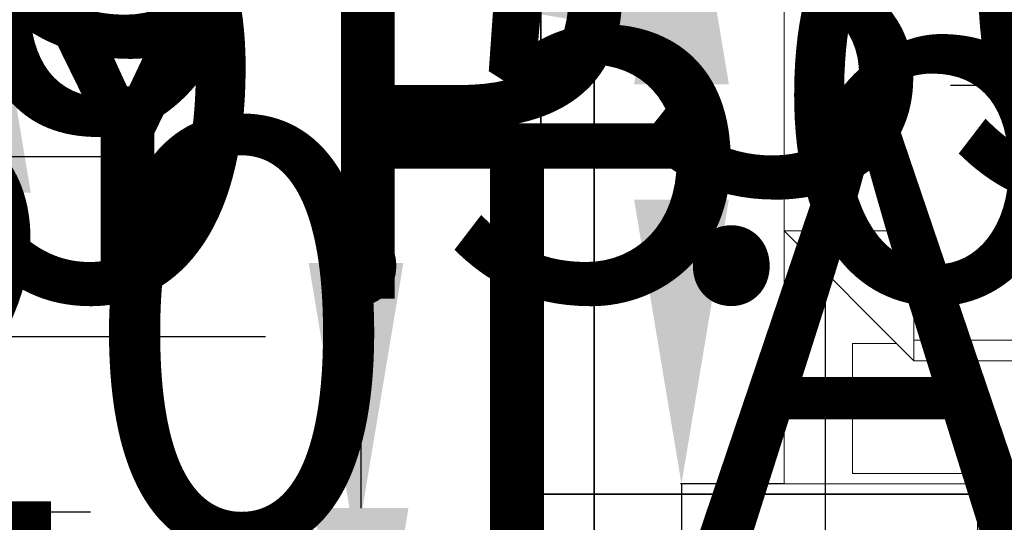
# Model space of a CAD drawing. Units: inches. Extents: x -307 to 2141, y -58 to 895.
# Tile 12 of 28: x 666 to 833, y 312 to 396. Entities that reach past the tile are written whole.
import ezdxf

# ---------------------------------------------------------------- set-up
doc = ezdxf.new("R2010")
doc.units = ezdxf.units.IN
doc.header["$MEASUREMENT"] = 0
for name, color, linetype, lineweight in [('A-ANNO-DIMS', 2, 'Continuous', 18), ('A-FURN', 8, 'Continuous', 18), ('A-WALL', 7, 'Continuous', 35)]:
    doc.layers.add(name, color=color, linetype=linetype, lineweight=lineweight)
doc.styles.get("Standard").update_dxf_attribs({"font": 'arial.ttf'})
doc.dimstyles.get("Standard").update_dxf_attribs({"dimtxt": 72, "dimasz": 48, "dimexe": 0.18, "dimexo": 0.0625, "dimgap": 0.09, "dimtad": 0, "dimtih": 1, "dimtoh": 1, "dimdec": 0, "dimrnd": 48, "dimzin": 0, "dimdsep": 46, "dimlunit": 3, "dimtxsty": 'Standard', "dimcen": 0.09, "dimadec": 0, "dimazin": 0, "dimtfac": 1, "dimtdec": 0, "dimtofl": 0, "dimtmove": 0, "dimatfit": 3, "dimfxl": 1, "dimtolj": 1, "dimtzin": 0, "dimarcsym": 0})

# ---------------------------------------------------------------- blocks, each defined once
blk = doc.blocks.new('Bed - Queen')
for p, q in [((0, -80.00003), (0, 0)), ((0, 0), (59.99999, 0)), ((59.99999, 0), (59.99999, -80.00003)), ((7.99999, -1.2), (28.79998, -1.2)), ((7.99999, -14.4), (7.99999, -1.2)), ((28.79998, -1.2), (28.79998, -14.4)), ((31.19999, -1.2), (51.99999, -1.2)), ((31.19999, -14.4), (31.19999, -1.2)), ((51.99999, -1.2), (51.99999, -16.4)), ((0, -14.4), (44.8, -14.4)), ((59.99999, -29.6), (44.8, -14.4)), ((44.8, -14.4), (44.8, -29.6)), ((44.8, -16.8), (0, -16.8)), ((51.99999, -16.4), (46.79936, -16.4)), ((44.8, -29.6), (59.99999, -29.6)), ((59.99999, -80.00003), (0, -80.00003))]:
    blk.add_line(p, q)
blk = doc.blocks.new('*D28')
at = {"layer": 'A-ANNO-DIMS', "color": 0, "lineweight": -2, "transparency": 16777216}
for p, q in [((795.36, 433.55), (777.92, 433.55)), ((778.1, 385.55), (778.1, 366.07)), ((795.36, 318.07), (777.92, 318.07)), ((778.1, 318.07), (778.1, 270.07)), ((778.1, 270.07), (730.1, 270.07))]:
    blk.add_line(p, q, dxfattribs=at)
at = {"layer": 'A-ANNO-DIMS', "color": 0, "transparency": 16777216}
for points in [[(770.1, 385.55), (786.1, 385.55), (778.1, 433.55)], [(770.1, 366.07), (786.1, 366.07), (778.1, 318.07)]]:
    blk.add_solid(points, dxfattribs=at)
at = {"layer": 'Defpoints', "color": 0, "transparency": 16777216}
for p in [(795.42, 433.55), (778.1, 318.07), (795.42, 318.07)]:
    blk.add_point(p, dxfattribs=at)
at = {"layer": 'A-ANNO-DIMS', "color": 0, "transparency": 16777216, "insert": (534.42, 270.07), "char_height": 72, "attachment_point": 5}
blk.add_mtext('\\A1;BED 115', dxfattribs=at)
blk = doc.blocks.new('*D30')
at = {"layer": 'A-ANNO-DIMS', "color": 0, "lineweight": -2, "transparency": 16777216}
for p, q in [((570.74, 532.83), (570.74, 580.83)), ((570.74, 580.83), (618.74, 580.83)), ((565.4, 484.83), (570.92, 484.83)), ((565.4, 448.83), (570.92, 448.83)), ((570.74, 400.83), (570.74, 352.83))]:
    blk.add_line(p, q, dxfattribs=at)
at = {"layer": 'A-ANNO-DIMS', "color": 0, "transparency": 16777216}
for points in [[(562.74, 532.83), (578.74, 532.83), (570.74, 484.83)], [(562.74, 400.83), (578.74, 400.83), (570.74, 448.83)]]:
    blk.add_solid(points, dxfattribs=at)
at = {"layer": 'Defpoints', "color": 0, "transparency": 16777216}
for p in [(565.34, 484.83), (570.74, 484.83), (565.34, 448.83)]:
    blk.add_point(p, dxfattribs=at)
at = {"layer": 'A-ANNO-DIMS', "color": 0, "transparency": 16777216, "insert": (1030.17, 580.83), "char_height": 72, "attachment_point": 5}
blk.add_mtext('\\A1;WINDOW 36 TYP.', dxfattribs=at)
blk = doc.blocks.new('*D31')
at = {"layer": 'A-ANNO-DIMS', "color": 0, "lineweight": -2, "transparency": 16777216}
for p, q in [((556.34, 448.77), (556.34, 443.25)), ((565.34, 448.77), (565.34, 443.25)), ((508.34, 443.43), (460.34, 443.43)), ((613.34, 443.43), (661.34, 443.43))]:
    blk.add_line(p, q, dxfattribs=at)
at = {"layer": 'A-ANNO-DIMS', "color": 0, "transparency": 16777216}
for points in [[(508.34, 451.43), (508.34, 435.43), (556.34, 443.43)], [(613.34, 451.43), (613.34, 435.43), (565.34, 443.43)]]:
    blk.add_solid(points, dxfattribs=at)
at = {"layer": 'Defpoints', "color": 0, "transparency": 16777216}
for p in [(556.34, 448.83), (565.34, 448.83), (565.34, 443.43)]:
    blk.add_point(p, dxfattribs=at)
at = {"layer": 'A-ANNO-DIMS', "color": 0, "transparency": 16777216, "insert": (808.69, 443.43), "char_height": 72, "attachment_point": 5}
blk.add_mtext('\\A1;9 TYP.', dxfattribs=at)
blk = doc.blocks.new('*D35')
at = {"layer": 'A-ANNO-DIMS', "color": 0, "lineweight": -2, "transparency": 16777216}
for p, q in [((907.34, 443.03), (907.34, 453.95)), ((916.34, 443.03), (916.34, 453.95)), ((859.34, 453.77), (811.34, 453.77)), ((964.34, 453.77), (1012.34, 453.77))]:
    blk.add_line(p, q, dxfattribs=at)
at = {"layer": 'A-ANNO-DIMS', "color": 0, "transparency": 16777216}
for points in [[(859.34, 461.77), (859.34, 445.77), (907.34, 453.77)], [(964.34, 461.77), (964.34, 445.77), (916.34, 453.77)]]:
    blk.add_solid(points, dxfattribs=at)
at = {"layer": 'Defpoints', "color": 0, "transparency": 16777216}
for p in [(907.34, 453.77), (907.34, 442.97), (916.34, 442.97)]:
    blk.add_point(p, dxfattribs=at)
at = {"layer": 'A-ANNO-DIMS', "color": 0, "transparency": 16777216, "insert": (663.98, 453.77), "char_height": 72, "attachment_point": 5}
blk.add_mtext('\\A1;9 TYP.', dxfattribs=at)
blk = doc.blocks.new('*D36')
at = {"layer": 'A-ANNO-DIMS', "color": 0, "lineweight": -2, "transparency": 16777216}
for p, q in [((871.71, 562.4), (871.76, 610.4)), ((876.55, 514.4), (871.47, 514.4)), ((876.51, 481.35), (871.44, 481.36)), ((871.56, 433.36), (871.51, 385.36)), ((871.51, 385.36), (823.51, 385.36))]:
    blk.add_line(p, q, dxfattribs=at)
at = {"layer": 'A-ANNO-DIMS', "color": 0, "transparency": 16777216}
for points in [[(863.71, 562.41), (879.71, 562.4), (871.65, 514.4)], [(863.56, 433.37), (879.56, 433.35), (871.62, 481.36)]]:
    blk.add_solid(points, dxfattribs=at)
at = {"layer": 'Defpoints', "color": 0, "transparency": 16777216}
for p in [(876.61, 514.4), (871.62, 481.36), (876.57, 481.35)]:
    blk.add_point(p, dxfattribs=at)
at = {"layer": 'A-ANNO-DIMS', "color": 0, "transparency": 16777216, "insert": (548.95, 385.36), "char_height": 72, "attachment_point": 5}
blk.add_mtext('\\A1;WC 33 TYP.', dxfattribs=at)
blk = doc.blocks.new('*D38')
at = {"layer": 'A-ANNO-DIMS', "color": 0, "lineweight": -2, "transparency": 16777216}
for p, q in [((646.5, 213.85), (646.5, 222.97)), ((706.5, 213.85), (706.5, 222.97)), ((598.5, 222.79), (550.5, 222.79)), ((754.5, 222.79), (802.5, 222.79))]:
    blk.add_line(p, q, dxfattribs=at)
at = {"layer": 'A-ANNO-DIMS', "color": 0, "transparency": 16777216}
for points in [[(598.5, 230.79), (598.5, 214.79), (646.5, 222.79)], [(754.5, 230.79), (754.5, 214.79), (706.5, 222.79)]]:
    blk.add_solid(points, dxfattribs=at)
at = {"layer": 'Defpoints', "color": 0, "transparency": 16777216}
for p in [(646.5, 222.79), (646.5, 213.79), (706.5, 213.79)]:
    blk.add_point(p, dxfattribs=at)
at = {"layer": 'A-ANNO-DIMS', "color": 0, "transparency": 16777216, "insert": (97.26, 222.79), "char_height": 72, "attachment_point": 5}
blk.add_mtext('\\A1;LOVESEAT 60 TYP.', dxfattribs=at)
blk = doc.blocks.new('*D41')
at = {"layer": 'A-ANNO-DIMS', "color": 0, "lineweight": -2, "transparency": 16777216}
for p, q in [((768.38, 207.13), (768.38, 255.13)), ((768.38, 255.13), (816.38, 255.13)), ((762.83, 159.13), (768.56, 159.13)), ((762.83, 128.96), (768.56, 128.96)), ((768.38, 80.96), (768.38, 32.96))]:
    blk.add_line(p, q, dxfattribs=at)
at = {"layer": 'A-ANNO-DIMS', "color": 0, "transparency": 16777216}
for points in [[(760.38, 207.13), (776.38, 207.13), (768.38, 159.13)], [(760.38, 80.96), (776.38, 80.96), (768.38, 128.96)]]:
    blk.add_solid(points, dxfattribs=at)
at = {"layer": 'Defpoints', "color": 0, "transparency": 16777216}
for p in [(762.77, 159.13), (768.38, 159.13), (762.77, 128.96)]:
    blk.add_point(p, dxfattribs=at)
at = {"layer": 'A-ANNO-DIMS', "color": 0, "transparency": 16777216, "insert": (991.68, 255.13), "char_height": 72, "attachment_point": 5}
blk.add_mtext('\\A1;30 TYP.', dxfattribs=at)
blk = doc.blocks.new('*D48')
at = {"layer": 'A-ANNO-DIMS', "color": 0, "lineweight": -2, "transparency": 16777216}
for p, q in [((724, 313.98), (724, 361.98)), ((732.94, 265.98), (723.82, 265.98)), ((732.94, 205.98), (723.82, 205.98)), ((724, 157.98), (724, 109.98)), ((724, 109.98), (676, 109.98))]:
    blk.add_line(p, q, dxfattribs=at)
at = {"layer": 'A-ANNO-DIMS', "color": 0, "transparency": 16777216}
for points in [[(716, 313.98), (732, 313.98), (724, 265.98)], [(716, 157.98), (732, 157.98), (724, 205.98)]]:
    blk.add_solid(points, dxfattribs=at)
at = {"layer": 'Defpoints', "color": 0, "transparency": 16777216}
for p in [(733, 265.98), (724, 205.98), (733, 205.98)]:
    blk.add_point(p, dxfattribs=at)
at = {"layer": 'A-ANNO-DIMS', "color": 0, "transparency": 16777216, "insert": (321.56, 109.98), "char_height": 72, "attachment_point": 5}
blk.add_mtext('\\A1;MEDIA UNIT 60', dxfattribs=at)
blk = doc.blocks.new('*D50')
at = {"layer": 'A-ANNO-DIMS', "color": 0, "lineweight": -2, "transparency": 16777216}
for p, q in [((565.34, 315.8), (565.34, 313.15)), ((582.27, 315.8), (582.27, 313.15)), ((517.34, 313.33), (469.34, 313.33)), ((630.27, 313.33), (678.27, 313.33))]:
    blk.add_line(p, q, dxfattribs=at)
at = {"layer": 'A-ANNO-DIMS', "color": 0, "transparency": 16777216}
for points in [[(517.34, 321.33), (517.34, 305.33), (565.34, 313.33)], [(630.27, 321.33), (630.27, 305.33), (582.27, 313.33)]]:
    blk.add_solid(points, dxfattribs=at)
at = {"layer": 'Defpoints', "color": 0, "transparency": 16777216}
for p in [(565.34, 315.87), (582.27, 315.87), (565.34, 313.33)]:
    blk.add_point(p, dxfattribs=at)
at = {"layer": 'A-ANNO-DIMS', "color": 0, "transparency": 16777216, "insert": (226.65, 313.33), "char_height": 72, "attachment_point": 5}
blk.add_mtext('\\A1;PHONE 17', dxfattribs=at)
blk = doc.blocks.new('*D51')
at = {"layer": 'A-ANNO-DIMS', "color": 0, "lineweight": -2, "transparency": 16777216}
for p, q in [((562.8, 379.11), (562.8, 427.11)), ((562.8, 427.11), (610.8, 427.11)), ((565.27, 331.11), (562.62, 331.11)), ((565.27, 315.87), (562.62, 315.87)), ((562.8, 267.87), (562.8, 219.87))]:
    blk.add_line(p, q, dxfattribs=at)
at = {"layer": 'A-ANNO-DIMS', "color": 0, "transparency": 16777216}
for points in [[(554.8, 379.11), (570.8, 379.11), (562.8, 331.11)], [(554.8, 267.87), (570.8, 267.87), (562.8, 315.87)]]:
    blk.add_solid(points, dxfattribs=at)
at = {"layer": 'Defpoints', "color": 0, "transparency": 16777216}
for p in [(562.8, 331.11), (565.34, 331.11), (565.34, 315.87)]:
    blk.add_point(p, dxfattribs=at)
at = {"layer": 'A-ANNO-DIMS', "color": 0, "transparency": 16777216, "insert": (659.34, 427.11), "char_height": 72, "attachment_point": 5}
blk.add_mtext('\\A1;15', dxfattribs=at)
blk = doc.blocks.new('*D52')
at = {"layer": 'A-ANNO-DIMS', "color": 0, "lineweight": -2, "transparency": 16777216}
for p, q in [((660.21, 554.25), (660.21, 602.25)), ((673.8, 506.25), (660.03, 506.25)), ((673.8, 415.25), (660.03, 415.25)), ((660.21, 367.25), (660.21, 319.25))]:
    blk.add_line(p, q, dxfattribs=at)
at = {"layer": 'A-ANNO-DIMS', "color": 0, "transparency": 16777216}
for points in [[(652.21, 554.25), (668.21, 554.25), (660.21, 506.25)], [(652.21, 367.25), (668.21, 367.25), (660.21, 415.25)]]:
    blk.add_solid(points, dxfattribs=at)
at = {"layer": 'Defpoints', "color": 0, "transparency": 16777216}
for p in [(673.86, 506.25), (660.21, 415.25), (673.86, 415.25)]:
    blk.add_point(p, dxfattribs=at)
at = {"layer": 'A-ANNO-DIMS', "color": 0, "transparency": 16777216, "insert": (660.21, 460.75), "char_height": 72, "attachment_point": 5}
blk.add_mtext('\\A1;DINING SET 91', dxfattribs=at)
blk = doc.blocks.new('*D53')
at = {"layer": 'A-ANNO-DIMS', "color": 0, "lineweight": -2, "transparency": 16777216}
for p, q in [((673.86, 415.19), (673.86, 401.42)), ((728.86, 415.19), (728.86, 401.42)), ((625.86, 401.6), (577.86, 401.6)), ((776.86, 401.6), (824.86, 401.6))]:
    blk.add_line(p, q, dxfattribs=at)
at = {"layer": 'A-ANNO-DIMS', "color": 0, "transparency": 16777216}
for points in [[(625.86, 409.6), (625.86, 393.6), (673.86, 401.6)], [(776.86, 409.6), (776.86, 393.6), (728.86, 401.6)]]:
    blk.add_solid(points, dxfattribs=at)
at = {"layer": 'Defpoints', "color": 0, "transparency": 16777216}
for p in [(673.86, 415.25), (728.86, 415.25), (728.86, 401.6)]:
    blk.add_point(p, dxfattribs=at)
at = {"layer": 'A-ANNO-DIMS', "color": 0, "transparency": 16777216, "insert": (876.79, 401.6), "char_height": 72, "attachment_point": 5}
blk.add_mtext('\\A1;55', dxfattribs=at)
blk = doc.blocks.new('*D54')
at = {"layer": 'A-ANNO-DIMS', "color": 0, "lineweight": -2, "transparency": 16777216}
for p, q in [((605.34, 412.35), (605.34, 460.35)), ((605.34, 460.35), (653.34, 460.35)), ((596.4, 364.35), (605.52, 364.35)), ((596.4, 304.35), (605.52, 304.35)), ((605.34, 256.35), (605.34, 208.35))]:
    blk.add_line(p, q, dxfattribs=at)
at = {"layer": 'A-ANNO-DIMS', "color": 0, "transparency": 16777216}
for points in [[(597.34, 412.35), (613.34, 412.35), (605.34, 364.35)], [(597.34, 256.35), (613.34, 256.35), (605.34, 304.35)]]:
    blk.add_solid(points, dxfattribs=at)
at = {"layer": 'Defpoints', "color": 0, "transparency": 16777216}
for p in [(596.34, 364.35), (605.34, 364.35), (596.34, 304.35)]:
    blk.add_point(p, dxfattribs=at)
at = {"layer": 'A-ANNO-DIMS', "color": 0, "transparency": 16777216, "insert": (854, 460.35), "char_height": 72, "attachment_point": 5}
blk.add_mtext('\\A1;DESK 60', dxfattribs=at)
blk = doc.blocks.new('*D55')
at = {"layer": 'A-ANNO-DIMS', "color": 0, "lineweight": -2, "transparency": 16777216}
for p, q in [((517.34, 373.35), (469.34, 373.35)), ((565.34, 364.41), (565.34, 373.53)), ((596.34, 364.41), (596.34, 373.53)), ((644.34, 373.35), (692.34, 373.35))]:
    blk.add_line(p, q, dxfattribs=at)
at = {"layer": 'A-ANNO-DIMS', "color": 0, "transparency": 16777216}
for points in [[(517.34, 381.35), (517.34, 365.35), (565.34, 373.35)], [(644.34, 381.35), (644.34, 365.35), (596.34, 373.35)]]:
    blk.add_solid(points, dxfattribs=at)
at = {"layer": 'Defpoints', "color": 0, "transparency": 16777216}
for p in [(565.34, 373.35), (565.34, 364.35), (596.34, 364.35)]:
    blk.add_point(p, dxfattribs=at)
at = {"layer": 'A-ANNO-DIMS', "color": 0, "transparency": 16777216, "insert": (424.65, 373.35), "char_height": 72, "attachment_point": 5}
blk.add_mtext('\\A1;31', dxfattribs=at)
blk = doc.blocks.new('*D58')
at = {"layer": 'A-ANNO-DIMS', "color": 0, "lineweight": -2, "transparency": 16777216}
for p, q in [((624.38, 334.8), (624.38, 382.8)), ((611.84, 286.8), (624.56, 286.8)), ((611.84, 202.8), (624.56, 202.8)), ((624.38, 154.8), (624.38, 106.8))]:
    blk.add_line(p, q, dxfattribs=at)
at = {"layer": 'A-ANNO-DIMS', "color": 0, "transparency": 16777216}
for points in [[(616.38, 334.8), (632.38, 334.8), (624.38, 286.8)], [(616.38, 154.8), (632.38, 154.8), (624.38, 202.8)]]:
    blk.add_solid(points, dxfattribs=at)
at = {"layer": 'Defpoints', "color": 0, "transparency": 16777216}
for p in [(611.78, 286.8), (624.38, 286.8), (611.78, 202.8)]:
    blk.add_point(p, dxfattribs=at)
at = {"layer": 'A-ANNO-DIMS', "color": 0, "transparency": 16777216, "insert": (624.38, 244.8), "char_height": 72, "attachment_point": 5}
blk.add_mtext('\\A1;SOFA 84', dxfattribs=at)
blk = doc.blocks.new('*D59')
at = {"layer": 'A-ANNO-DIMS', "color": 0, "lineweight": -2, "transparency": 16777216}
for p, q in [((527.11, 299.4), (479.11, 299.4)), ((575.11, 286.86), (575.11, 299.58)), ((611.78, 286.86), (611.78, 299.58)), ((659.78, 299.4), (707.78, 299.4))]:
    blk.add_line(p, q, dxfattribs=at)
at = {"layer": 'A-ANNO-DIMS', "color": 0, "transparency": 16777216}
for points in [[(527.11, 307.4), (527.11, 291.4), (575.11, 299.4)], [(659.78, 307.4), (659.78, 291.4), (611.78, 299.4)]]:
    blk.add_solid(points, dxfattribs=at)
at = {"layer": 'Defpoints', "color": 0, "transparency": 16777216}
for p in [(575.11, 299.4), (575.11, 286.8), (611.78, 286.8)]:
    blk.add_point(p, dxfattribs=at)
at = {"layer": 'A-ANNO-DIMS', "color": 0, "transparency": 16777216, "insert": (427.48, 299.4), "char_height": 72, "attachment_point": 5}
blk.add_mtext('\\A1;37', dxfattribs=at)
blk = doc.blocks.new('*D60')
at = {"layer": 'A-ANNO-DIMS', "color": 0, "lineweight": -2, "transparency": 16777216}
for p, q in [((659.86, 294.95), (659.86, 342.95)), ((659.86, 342.95), (707.86, 342.95)), ((663.34, 246.95), (659.68, 246.95)), ((663.34, 223.32), (659.68, 223.32)), ((659.86, 175.32), (659.86, 127.32))]:
    blk.add_line(p, q, dxfattribs=at)
at = {"layer": 'A-ANNO-DIMS', "color": 0, "transparency": 16777216}
for points in [[(651.86, 294.95), (667.86, 294.95), (659.86, 246.95)], [(651.86, 175.32), (667.86, 175.32), (659.86, 223.32)]]:
    blk.add_solid(points, dxfattribs=at)
at = {"layer": 'Defpoints', "color": 0, "transparency": 16777216}
for p in [(659.86, 246.95), (663.4, 246.95), (663.4, 223.32)]:
    blk.add_point(p, dxfattribs=at)
at = {"layer": 'A-ANNO-DIMS', "color": 0, "transparency": 16777216, "insert": (933.57, 342.95), "char_height": 72, "attachment_point": 5}
blk.add_mtext('\\A1;TABLE 24', dxfattribs=at)
blk = doc.blocks.new('*D63')
at = {"layer": 'A-ANNO-DIMS', "color": 0, "lineweight": -2, "transparency": 16777216}
for p, q in [((916.4, 691.34), (947.72, 691.34)), ((947.54, 643.34), (947.54, 416.19)), ((947.54, 115.34), (947.54, 342.49)), ((704.68, 67.34), (947.72, 67.34))]:
    blk.add_line(p, q, dxfattribs=at)
at = {"layer": 'A-ANNO-DIMS', "color": 0, "transparency": 16777216}
for points in [[(939.54, 643.34), (955.54, 643.34), (947.54, 691.34)], [(939.54, 115.34), (955.54, 115.34), (947.54, 67.34)]]:
    blk.add_solid(points, dxfattribs=at)
at = {"layer": 'Defpoints', "color": 0, "transparency": 16777216}
for p in [(916.34, 691.34), (704.62, 67.34), (947.54, 67.34)]:
    blk.add_point(p, dxfattribs=at)
at = {"layer": 'A-ANNO-DIMS', "color": 0, "transparency": 16777216, "insert": (947.54, 379.34), "char_height": 72, "attachment_point": 5}
blk.add_mtext('\\A1;624', dxfattribs=at)
blk = doc.blocks.new('*D68')
at = {"layer": 'A-ANNO-DIMS', "color": 0, "lineweight": -2, "transparency": 16777216}
for p, q in [((525.13, 586.34), (525.13, 634.34)), ((525.13, 634.34), (573.13, 634.34)), ((565.27, 538.34), (524.95, 538.34)), ((556.27, 484.83), (524.95, 484.83)), ((525.13, 436.83), (525.13, 388.83))]:
    blk.add_line(p, q, dxfattribs=at)
at = {"layer": 'A-ANNO-DIMS', "color": 0, "transparency": 16777216}
for points in [[(517.13, 586.34), (533.13, 586.34), (525.13, 538.34)], [(517.13, 436.83), (533.13, 436.83), (525.13, 484.83)]]:
    blk.add_solid(points, dxfattribs=at)
at = {"layer": 'Defpoints', "color": 0, "transparency": 16777216}
for p in [(525.13, 538.34), (565.34, 538.34), (556.34, 484.83)]:
    blk.add_point(p, dxfattribs=at)
at = {"layer": 'A-ANNO-DIMS', "color": 0, "transparency": 16777216, "insert": (687.75, 634.34), "char_height": 72, "attachment_point": 5}
blk.add_mtext('\\A1;53.51', dxfattribs=at)
blk = doc.blocks.new('*D82')
at = {"layer": 'A-ANNO-DIMS', "color": 0, "lineweight": -2, "transparency": 16777216}
for p, q in [((525.13, 565.34), (525.13, 613.34)), ((525.13, 613.34), (573.13, 613.34)), ((802.27, 517.34), (524.95, 517.34)), ((802.27, 481.34), (524.95, 481.34)), ((525.13, 433.34), (525.13, 385.34))]:
    blk.add_line(p, q, dxfattribs=at)
at = {"layer": 'A-ANNO-DIMS', "color": 0, "transparency": 16777216}
for points in [[(517.13, 565.34), (533.13, 565.34), (525.13, 517.34)], [(517.13, 433.34), (533.13, 433.34), (525.13, 481.34)]]:
    blk.add_solid(points, dxfattribs=at)
at = {"layer": 'Defpoints', "color": 0, "transparency": 16777216}
for p in [(525.13, 517.34), (802.34, 517.34), (802.34, 481.34)]:
    blk.add_point(p, dxfattribs=at)
at = {"layer": 'A-ANNO-DIMS', "color": 0, "transparency": 16777216, "insert": (624.74, 613.34), "char_height": 72, "attachment_point": 5}
blk.add_mtext('\\A1;36', dxfattribs=at)
blk = doc.blocks.new('*D83')
at = {"layer": 'A-ANNO-DIMS', "color": 0, "lineweight": -2, "transparency": 16777216}
for p, q in [((947.54, 538.9), (947.54, 586.9)), ((916.4, 490.9), (947.72, 490.9)), ((907.4, 481.34), (947.72, 481.34)), ((947.54, 433.34), (947.54, 385.34)), ((947.54, 385.34), (899.54, 385.34))]:
    blk.add_line(p, q, dxfattribs=at)
at = {"layer": 'A-ANNO-DIMS', "color": 0, "transparency": 16777216}
for points in [[(939.54, 538.9), (955.54, 538.9), (947.54, 490.9)], [(939.54, 433.34), (955.54, 433.34), (947.54, 481.34)]]:
    blk.add_solid(points, dxfattribs=at)
at = {"layer": 'Defpoints', "color": 0, "transparency": 16777216}
for p in [(916.34, 490.9), (907.34, 481.34), (947.54, 481.34)]:
    blk.add_point(p, dxfattribs=at)
at = {"layer": 'A-ANNO-DIMS', "color": 0, "transparency": 16777216, "insert": (777.97, 385.34), "char_height": 72, "attachment_point": 5}
blk.add_mtext('\\A1;9.563', dxfattribs=at)
blk = doc.blocks.new('*D84')
at = {"layer": 'A-ANNO-DIMS', "color": 0, "lineweight": -2, "transparency": 16777216}
for p, q in [((763.34, 472.28), (763.34, 35.96)), ((907.34, 472.28), (907.34, 35.96)), ((811.34, 36.14), (859.34, 36.14)), ((907.34, 36.14), (955.34, 36.14))]:
    blk.add_line(p, q, dxfattribs=at)
at = {"layer": 'A-ANNO-DIMS', "color": 0, "transparency": 16777216}
for points in [[(811.34, 44.14), (811.34, 28.14), (763.34, 36.14)], [(859.34, 44.14), (859.34, 28.14), (907.34, 36.14)]]:
    blk.add_solid(points, dxfattribs=at)
at = {"layer": 'Defpoints', "color": 0, "transparency": 16777216}
for p in [(763.34, 472.34), (907.34, 472.34), (907.34, 36.14)]:
    blk.add_point(p, dxfattribs=at)
at = {"layer": 'A-ANNO-DIMS', "color": 0, "transparency": 16777216, "insert": (1031.43, 36.14), "char_height": 72, "attachment_point": 5}
blk.add_mtext('\\A1;144', dxfattribs=at)
blk = doc.blocks.new('*D88')
at = {"layer": 'A-ANNO-DIMS', "color": 0, "lineweight": -2, "transparency": 16777216}
for p, q in [((517.33584, 722.544828), (469.33584, 722.544828)), ((565.33584, 295.403328), (565.33584, 722.724828)), ((754.33584, 271.403328), (754.33584, 722.724828)), ((802.33584, 722.544828), (850.33584, 722.544828))]:
    blk.add_line(p, q, dxfattribs=at)
at = {"layer": 'A-ANNO-DIMS', "color": 0, "transparency": 16777216}
for points in [[(517.33584, 730.544828), (517.33584, 714.544828), (565.33584, 722.544828)], [(802.33584, 730.544828), (802.33584, 714.544828), (754.33584, 722.544828)]]:
    blk.add_solid(points, dxfattribs=at)
at = {"layer": 'Defpoints', "color": 0, "transparency": 16777216}
for p in [(754.33584, 722.544828), (565.33584, 295.340828), (754.33584, 271.340828)]:
    blk.add_point(p, dxfattribs=at)
at = {"layer": 'A-ANNO-DIMS', "color": 0, "transparency": 16777216, "insert": (659.83584, 722.544828), "char_height": 72, "attachment_point": 5}
blk.add_mtext('\\A1;189', dxfattribs=at)
blk = doc.blocks.new('*D89')
at = {"layer": 'A-ANNO-DIMS', "color": 0, "lineweight": -2, "transparency": 16777216}
for p, q in [((525.13, 295.34), (525.13, 343.34)), ((525.13, 343.34), (573.13, 343.34)), ((565.27, 295.34), (524.95, 295.34)), ((525.13, 223.34), (525.13, 247.34)), ((556.27, 175.34), (524.95, 175.34))]:
    blk.add_line(p, q, dxfattribs=at)
at = {"layer": 'A-ANNO-DIMS', "color": 0, "transparency": 16777216}
for points in [[(517.13, 247.34), (533.13, 247.34), (525.13, 295.34)], [(517.13, 223.34), (533.13, 223.34), (525.13, 175.34)]]:
    blk.add_solid(points, dxfattribs=at)
at = {"layer": 'Defpoints', "color": 0, "transparency": 16777216}
for p in [(525.13, 295.34), (565.34, 295.34), (556.34, 175.34)]:
    blk.add_point(p, dxfattribs=at)
at = {"layer": 'A-ANNO-DIMS', "color": 0, "transparency": 16777216, "insert": (649.25, 343.34), "char_height": 72, "attachment_point": 5}
blk.add_mtext('\\A1;120', dxfattribs=at)
blk = doc.blocks.new('*D99')
at = {"layer": 'A-ANNO-DIMS', "color": 0, "lineweight": -2, "transparency": 16777216}
for p, q in [((763.34, 481.28), (763.34, 35.96)), ((802.34, 481.28), (802.34, 35.96)), ((715.34, 36.14), (667.34, 36.14)), ((850.34, 36.14), (898.34, 36.14))]:
    blk.add_line(p, q, dxfattribs=at)
at = {"layer": 'A-ANNO-DIMS', "color": 0, "transparency": 16777216}
for points in [[(715.34, 44.14), (715.34, 28.14), (763.34, 36.14)], [(850.34, 44.14), (850.34, 28.14), (802.34, 36.14)]]:
    blk.add_solid(points, dxfattribs=at)
at = {"layer": 'Defpoints', "color": 0, "transparency": 16777216}
for p in [(763.34, 481.34), (802.34, 481.34), (802.34, 36.14)]:
    blk.add_point(p, dxfattribs=at)
at = {"layer": 'A-ANNO-DIMS', "color": 0, "transparency": 16777216, "insert": (950.04, 36.14), "char_height": 72, "attachment_point": 5}
blk.add_mtext('\\A1;39', dxfattribs=at)
blk = doc.blocks.new('*D100')
at = {"layer": 'A-ANNO-DIMS', "color": 0, "lineweight": -2, "transparency": 16777216}
for p, q in [((589.34, 409.28), (589.34, 35.96)), ((625.34, 409.28), (625.34, 35.96)), ((541.34, 36.14), (493.34, 36.14)), ((673.34, 36.14), (721.34, 36.14))]:
    blk.add_line(p, q, dxfattribs=at)
at = {"layer": 'A-ANNO-DIMS', "color": 0, "transparency": 16777216}
for points in [[(541.34, 44.14), (541.34, 28.14), (589.34, 36.14)], [(673.34, 44.14), (673.34, 28.14), (625.34, 36.14)]]:
    blk.add_solid(points, dxfattribs=at)
at = {"layer": 'Defpoints', "color": 0, "transparency": 16777216}
for p in [(589.34, 409.34), (625.34, 409.34), (625.34, 36.14)]:
    blk.add_point(p, dxfattribs=at)
at = {"layer": 'A-ANNO-DIMS', "color": 0, "transparency": 16777216, "insert": (772.95, 36.14), "char_height": 72, "attachment_point": 5}
blk.add_mtext('\\A1;36', dxfattribs=at)
blk = doc.blocks.new('*D105')
at = {"layer": 'A-ANNO-DIMS', "color": 0, "lineweight": -2, "transparency": 16777216}
for p, q in [((828.13, 271.34), (828.13, 319.34)), ((828.13, 319.34), (876.13, 319.34)), ((859.27, 223.34), (827.95, 223.34)), ((859.27, 211.34), (827.95, 211.34)), ((828.13, 163.34), (828.13, 115.34))]:
    blk.add_line(p, q, dxfattribs=at)
at = {"layer": 'A-ANNO-DIMS', "color": 0, "transparency": 16777216}
for points in [[(820.13, 271.34), (836.13, 271.34), (828.13, 223.34)], [(820.13, 163.34), (836.13, 163.34), (828.13, 211.34)]]:
    blk.add_solid(points, dxfattribs=at)
at = {"layer": 'Defpoints', "color": 0, "transparency": 16777216}
for p in [(828.13, 223.34), (859.34, 223.34), (859.34, 211.34)]:
    blk.add_point(p, dxfattribs=at)
at = {"layer": 'A-ANNO-DIMS', "color": 0, "transparency": 16777216, "insert": (924.03, 319.34), "char_height": 72, "attachment_point": 5}
blk.add_mtext('\\A1;12', dxfattribs=at)
blk = doc.blocks.new('*D108')
at = {"layer": 'A-ANNO-DIMS', "color": 0, "lineweight": -2, "transparency": 16777216}
for p, q in [((947.54, 550.66), (947.54, 598.66)), ((589.4, 502.66), (947.72, 502.66)), ((589.4, 409.34), (947.72, 409.34)), ((947.54, 361.34), (947.54, 313.34))]:
    blk.add_line(p, q, dxfattribs=at)
at = {"layer": 'A-ANNO-DIMS', "color": 0, "transparency": 16777216}
for points in [[(939.54, 550.66), (955.54, 550.66), (947.54, 502.66)], [(939.54, 361.34), (955.54, 361.34), (947.54, 409.34)]]:
    blk.add_solid(points, dxfattribs=at)
at = {"layer": 'Defpoints', "color": 0, "transparency": 16777216}
for p in [(589.34, 502.66), (947.54, 502.66), (589.34, 409.34)]:
    blk.add_point(p, dxfattribs=at)
at = {"layer": 'A-ANNO-DIMS', "color": 0, "transparency": 16777216, "insert": (947.54, 456), "char_height": 72, "attachment_point": 5}
blk.add_mtext('\\A1;93.32', dxfattribs=at)
blk = doc.blocks.new('*D109')
at = {"layer": 'A-ANNO-DIMS', "color": 0, "lineweight": -2, "transparency": 16777216}
for p, q in [((723.13, 355.34), (723.13, 403.34)), ((723.13, 403.34), (771.13, 403.34)), ((754.27, 307.34), (722.95, 307.34)), ((754.27, 271.34), (722.95, 271.34)), ((723.13, 223.34), (723.13, 175.34))]:
    blk.add_line(p, q, dxfattribs=at)
at = {"layer": 'A-ANNO-DIMS', "color": 0, "transparency": 16777216}
for points in [[(715.13, 355.34), (731.13, 355.34), (723.13, 307.34)], [(715.13, 223.34), (731.13, 223.34), (723.13, 271.34)]]:
    blk.add_solid(points, dxfattribs=at)
at = {"layer": 'Defpoints', "color": 0, "transparency": 16777216}
for p in [(723.13, 307.34), (754.34, 307.34), (754.34, 271.34)]:
    blk.add_point(p, dxfattribs=at)
at = {"layer": 'A-ANNO-DIMS', "color": 0, "transparency": 16777216, "insert": (822.74, 403.34), "char_height": 72, "attachment_point": 5}
blk.add_mtext('\\A1;36', dxfattribs=at)

msp = doc.modelspace()

# ---------------------------------------------------------------- linework, layer by layer
at = {"layer": 'A-WALL'}
for p, q in [((754.3358, 307.3408), (754.3358, 481.3408)), ((754.3358, 307.3408), (754.3358, 481.3408)), ((763.3358, 307.3408), (763.3358, 481.3408)), ((763.3358, 307.3408), (763.3358, 481.3408)), ((916.3358, 316.3408), (754.3358, 316.3408))]:
    msp.add_line(p, q, dxfattribs=at)

# ---------------------------------------------------------------- block references
at = {"layer": 'A-FURN', "xscale": 1.443457686913744, "yscale": 1.443457686913744, "zscale": 1.443457686913744, "rotation": 179.9999999999998}
msp.add_blockref('Bed - Queen', (882.0282, 318.073), dxfattribs=at)

# ---------------------------------------------------------------- dimensions: what is measured, and where the dimension line sits
at = {"layer": 'A-ANNO-DIMS'}
for base, p1, p2, picture, middle in [((754.3358, 722.5448), (565.3358, 295.3408), (754.3358, 271.3408), '*D88', (659.8358, 722.5448)), ((802.3358, 36.1368), (763.3358, 481.3408), (802.3358, 481.3408), '*D99', (950.0438, 36.1368)), ((907.3358, 36.1368), (763.3358, 472.3408), (907.3358, 472.3408), '*D84', (1031.4286, 36.1368)), ((728.8583, 401.5985), (673.8583, 415.2485), (728.8583, 415.2485), '*D53', (876.7874, 401.5985)), ((625.3358, 36.1368), (589.339, 409.3408), (625.3358, 409.3408), '*D100', (772.9456, 36.1368))]:
    dim = msp.add_linear_dim(base=base, p1=p1, p2=p2, dimstyle='Standard', override={"dimdec": 0, "dimlfac": 1, "dimrnd": 0, "dimzin": 0, "dimdsep": 46, "dimlunit": 2}, dxfattribs=at)
    dim.commit()
    dim.dimension.update_dxf_attribs({"geometry": picture, "text_midpoint": middle})
for base, p1, p2, angle, text, picture, middle in [((570.7358, 484.8333), (565.3358, 448.8333), (565.3358, 484.8333), 90, 'WINDOW <> TYP.', '*D30', (1030.1737, 580.8333)), ((660.2083, 415.2485), (673.8583, 506.2485), (673.8583, 415.2485), 270, 'DINING SET <>', '*D52', (660.2083, 460.7485)), ((871.6167, 481.3581), (876.6106, 514.3988), (876.5736, 481.3526), 269.935892, 'WC <> TYP.', '*D36', (548.95, 385.3582)), ((605.3358, 364.3488), (596.3358, 304.3488), (596.3358, 364.3488), 90, 'DESK <>', '*D54', (854.0043, 460.3488)), ((907.3358, 453.7692), (916.3358, 442.9669), (907.3358, 442.9669), 180, '<> TYP.', '*D35', (663.9798, 453.7692)), ((659.8571, 246.9465), (663.4018, 223.3153), (663.4018, 246.9465), 90, 'TABLE <>', '*D60', (933.5733, 342.9465)), ((778.0993, 318.073), (795.4208, 433.5496), (795.4208, 318.073), 270, 'BED <>', '*D28', (534.4158, 270.073)), ((565.3358, 313.3263), (582.2714, 315.8666), (565.3358, 315.8666), 180, 'PHONE <>', '*D50', (226.651, 313.3263)), ((646.4965, 222.7908), (706.4965, 213.7908), (646.4965, 213.7908), 180, 'LOVESEAT <> TYP.', '*D38', (97.2632, 222.7908)), ((624.377, 286.7976), (611.777, 202.7976), (611.777, 286.7976), 90, 'SOFA <>', '*D58', (624.377, 244.7976)), ((768.3792, 159.1282), (762.7703, 128.9569), (762.7703, 159.1282), 90, '<> TYP.', '*D41', (991.6806, 255.1282)), ((724.0025, 205.9815), (733.0025, 265.9815), (733.0025, 205.9815), 270, 'MEDIA UNIT <>', '*D48', (321.5605, 109.9815))]:
    dim = msp.add_linear_dim(base=base, p1=p1, p2=p2, angle=angle, text=text, dimstyle='Standard', override={"dimdec": 0, "dimlfac": 1, "dimrnd": 0, "dimzin": 0, "dimdsep": 46, "dimlunit": 2}, dxfattribs=at)
    dim.commit()
    dim.dimension.update_dxf_attribs({"geometry": picture, "text_midpoint": middle})
for base, p1, p2, angle, override, picture, middle in [((947.5398, 67.3408), (916.3358, 691.3408), (704.6211, 67.3408), 90, {"dimdec": 0, "dimlfac": 1, "dimrnd": 0, "dimzin": 0, "dimdsep": 46, "dimlunit": 2}, '*D63', (947.5398, 379.3408)), ((525.1318, 538.3408), (556.3358, 484.8333), (565.3358, 538.3408), 90, {"dimdec": 2, "dimlfac": 1, "dimrnd": 0, "dimzin": 0, "dimdsep": 46, "dimlunit": 2}, '*D68', (687.7539, 634.3408)), ((525.1318, 517.3408), (802.3358, 481.3408), (802.3358, 517.3408), 90, {"dimdec": 0, "dimlfac": 1, "dimrnd": 0, "dimzin": 0, "dimdsep": 46, "dimlunit": 2}, '*D82', (624.7416, 613.3408)), ((947.5398, 502.6632), (589.339, 409.3408), (589.339, 502.6632), 90, {"dimdec": 2, "dimlfac": 1, "dimrnd": 0, "dimzin": 0, "dimdsep": 46, "dimlunit": 2}, '*D108', (947.5398, 456.002)), ((947.5398, 481.3408), (916.3358, 490.9034), (907.3358, 481.3408), 90, {"dimdec": 3, "dimlfac": 1, "dimrnd": 0, "dimzin": 0, "dimdsep": 46, "dimlunit": 2}, '*D83', (777.9683, 385.3408)), ((562.7955, 331.1086), (565.3358, 315.8666), (565.3358, 331.1086), 90, {"dimdec": 0, "dimlfac": 1, "dimrnd": 0, "dimzin": 0, "dimdsep": 46, "dimlunit": 2}, '*D51', (659.3357, 427.1086)), ((723.1318, 307.3408), (754.3358, 271.3408), (754.3358, 307.3408), 90, {"dimdec": 0, "dimlfac": 1, "dimrnd": 0, "dimzin": 0, "dimdsep": 46, "dimlunit": 2}, '*D109', (822.7416, 403.3408)), ((565.3358, 373.3488), (596.3358, 364.3488), (565.3358, 364.3488), 180, {"dimdec": 0, "dimlfac": 1, "dimrnd": 0, "dimzin": 0, "dimdsep": 46, "dimlunit": 2}, '*D55', (424.651, 373.3488)), ((525.1318, 295.3408), (556.3358, 175.3408), (565.3358, 295.3408), 90, {"dimdec": 0, "dimlfac": 1, "dimrnd": 0, "dimzin": 0, "dimdsep": 46, "dimlunit": 2}, '*D89', (649.2491, 343.3408)), ((828.1318, 223.3408), (859.3358, 211.3408), (859.3358, 223.3408), 90, {"dimdec": 0, "dimlfac": 1, "dimrnd": 0, "dimzin": 0, "dimdsep": 46, "dimlunit": 2}, '*D105', (924.0336, 319.3408)), ((575.1104, 299.3976), (611.777, 286.7976), (575.1104, 286.7976), 180, {"dimdec": 0, "dimlfac": 1, "dimrnd": 0, "dimzin": 0, "dimdsep": 46, "dimlunit": 2}, '*D59', (427.476, 299.3976))]:
    dim = msp.add_linear_dim(base=base, p1=p1, p2=p2, angle=angle, dimstyle='Standard', override=override, dxfattribs=at)
    dim.commit()
    dim.dimension.update_dxf_attribs({"geometry": picture, "text_midpoint": middle})
dim = msp.add_linear_dim(base=(565.3358, 443.4333), p1=(556.3358, 448.8333), p2=(565.3358, 448.8333), text='<> TYP.', dimstyle='Standard', override={"dimdec": 0, "dimlfac": 1, "dimrnd": 0, "dimzin": 0, "dimdsep": 46, "dimlunit": 2}, dxfattribs=at)
dim.commit()
dim.dimension.update_dxf_attribs({"geometry": '*D31', "text_midpoint": (808.6919, 443.4333)})

doc.saveas('drawing.dxf')
